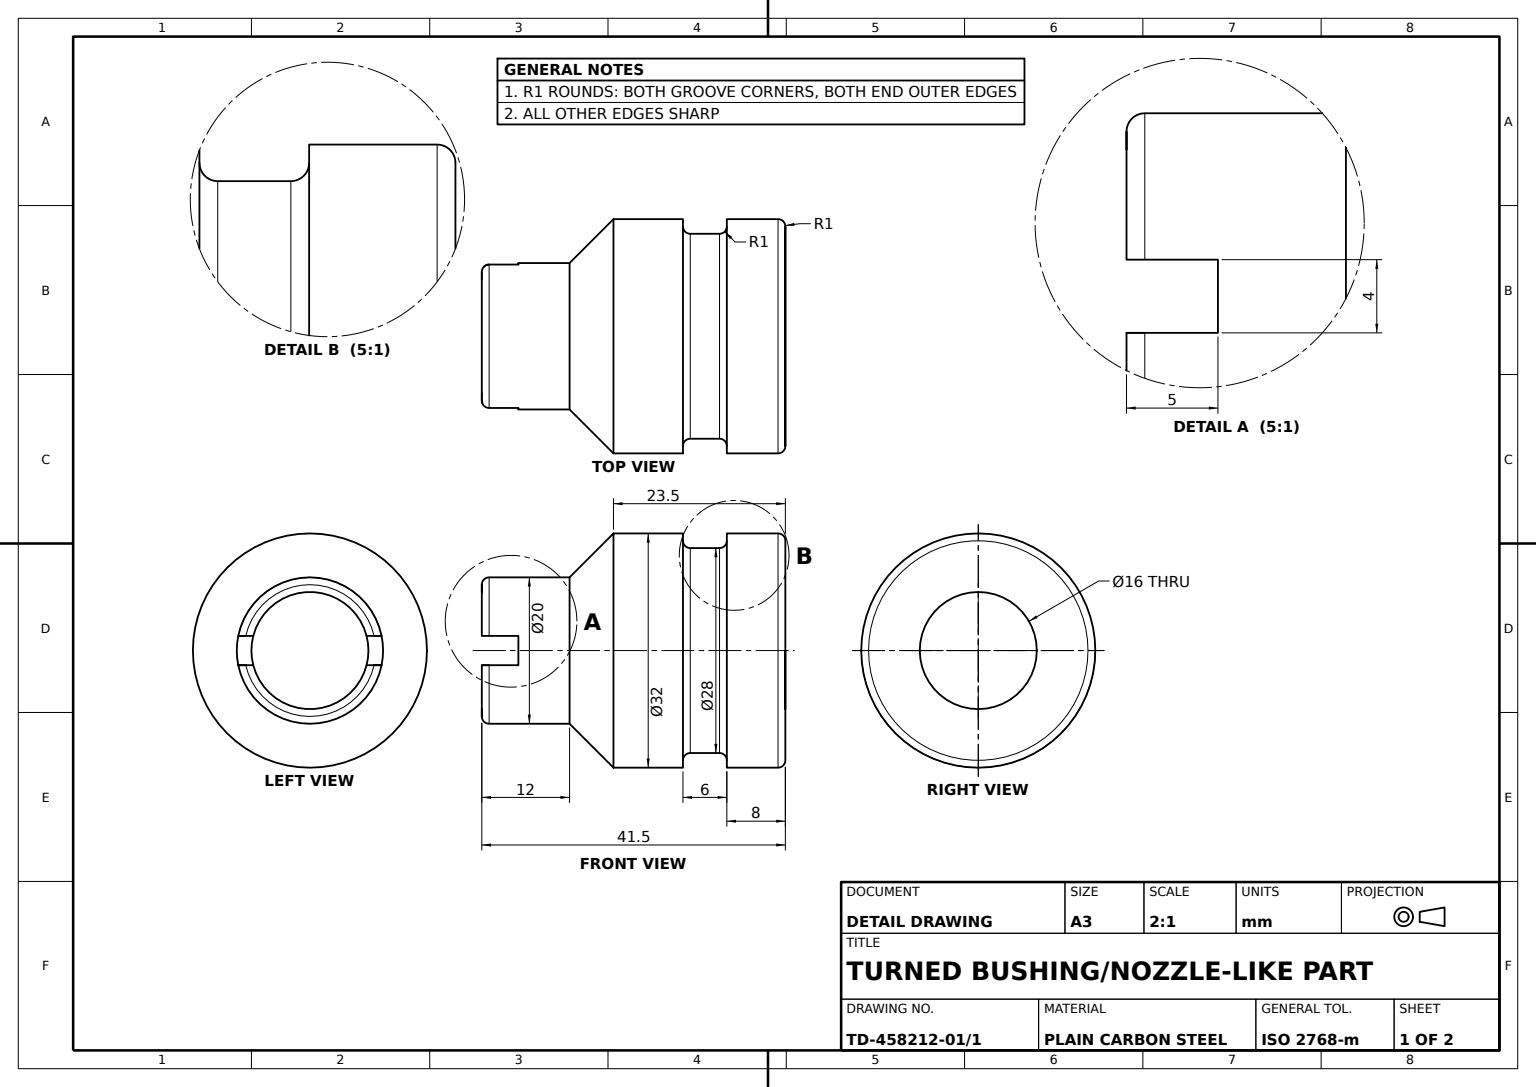
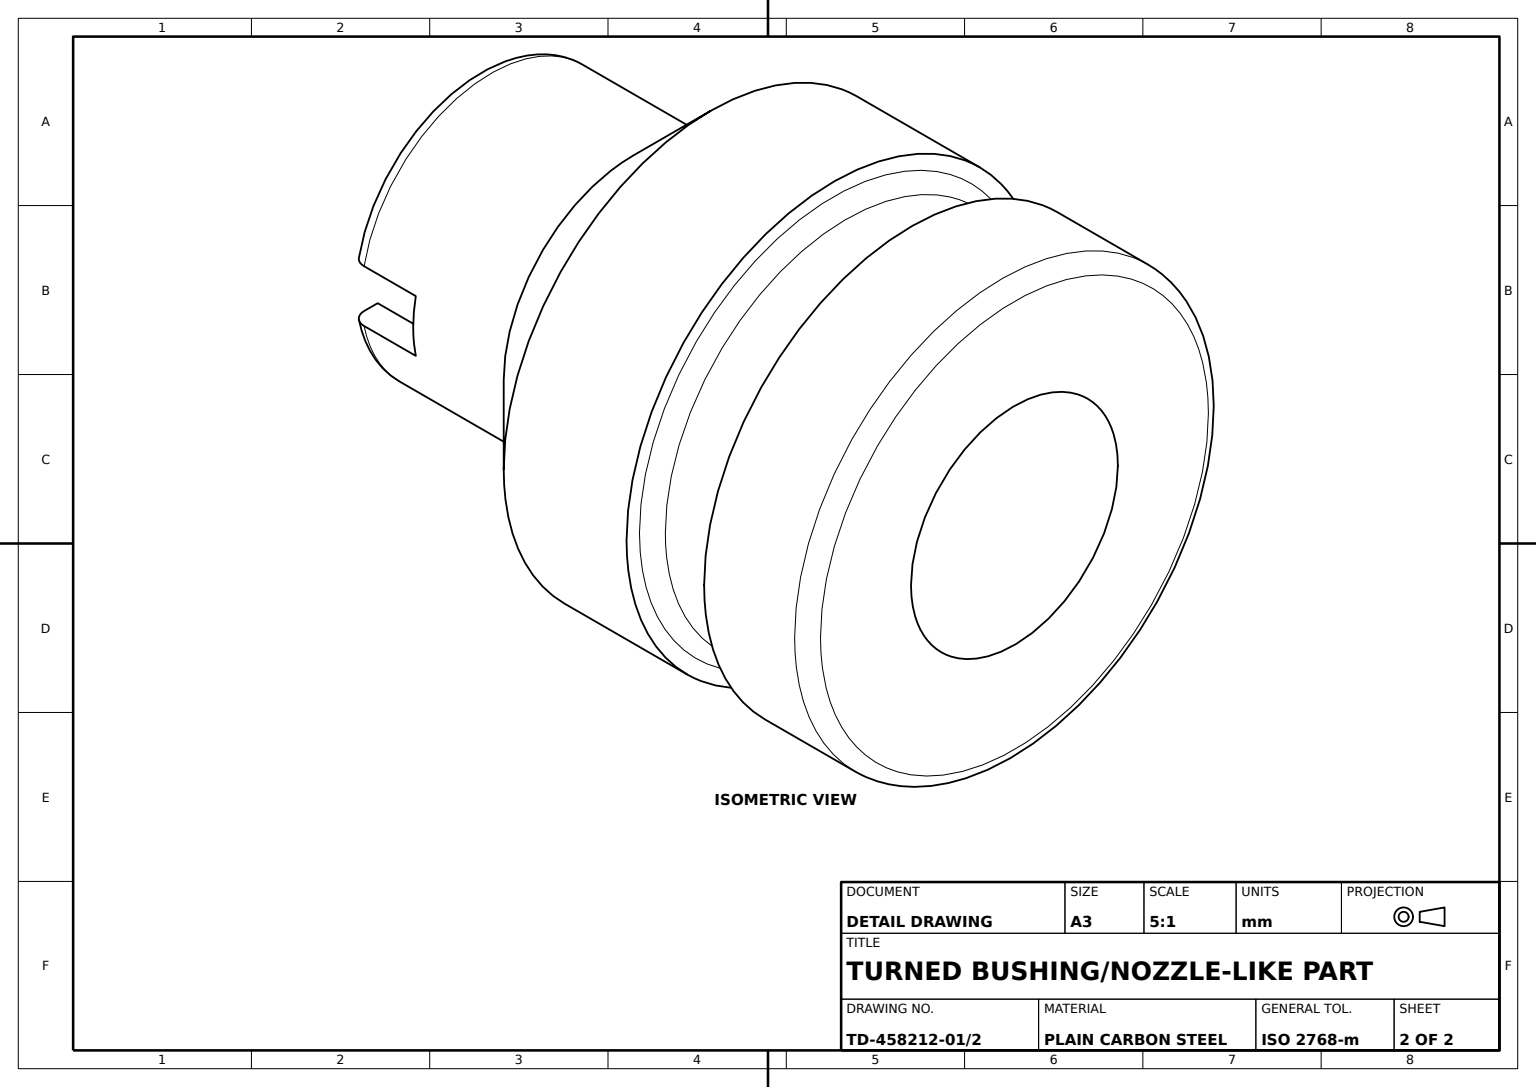
SolidWorks part; units mm, degrees
material "Plain Carbon Steel"
ref_plane "Front Plane" through (0, 0, 0) normal (0, 0, 1) x (1, 0, 0)
ref_plane "Top Plane" through (0, 0, 0) normal (0, 1, 0) x (1, 0, 0)
ref_plane "Right Plane" through (0, 0, 0) normal (1, 0, 0) x (0, 0, -1)
sketch "Bushing Revolve Profile" plane through (0, 0, 0) normal (0, 0, 1) x (1, 0, 0)
  line L0 (-18.7544, 8) -> (67.7711, 8) construction
  line L1 (0, 0) -> (0, -1)
  line L2 (1, -2) -> (12, -2)
  line L3 (12, -2) -> (18, -8)
  line L4 (18, -8) -> (27.5, -8)
  line L5 (27.5, -8) -> (27.5, -7)
  line L6 (28.5, -6) -> (32.5, -6)
  line L7 (33.5, -7) -> (33.5, -8)
  line L8 (33.5, -8) -> (40.5, -8)
  line L9 (41.5, -7) -> (41.5, 0)
  line L10 (0, 0) -> (41.5, 0)
  arc A0 (0, -1) -> (1, -2) centre (1, -1) ccw
  arc A1 (40.5, -8) -> (41.5, -7) centre (40.5, -7) ccw
  arc A2 (32.5, -6) -> (33.5, -7) centre (32.5, -7) cw
  arc A3 (27.5, -7) -> (28.5, -6) centre (28.5, -7) cw
  point P1 (30.5, -6)
  point P16 (41.5, -8)
  point P19 (33.5, -6)
  point P25 (27.5, -6)
  dimension "D9" = 1
  dimension "D1" = 41.5
  dimension "D2" = 12
  dimension "D3" = 8
  dimension "D4" = 6
  dimension "D5" = 23.5
  dimension "D6" = 135
  dimension "D7" = 8
  dimension "D8" = 14
  dimension "D10" = 16
revolve "Stepped Bushing Body" add sketch "Bushing Revolve Profile" angle 360 about L0
sketch "End Slot Profile" plane through (0, 0, 0) normal (0, 0, 1) x (1, 0, 0)
  line L0 (0, 8) -> (52.3679, 8) construction
  line L1 (0, 17) -> (0, -1) construction
  line L2 (0, 10) -> (5, 10)
  line L3 (5, 10) -> (5, 6)
  line L4 (5, 6) -> (0, 6)
  line L5 (0, 6) -> (0, 10)
  dimension "D1" = 4
  dimension "D2" = 5
extrude "End Slot Cut" cut sketch "End Slot Profile" against normal through all both and the other way through all
